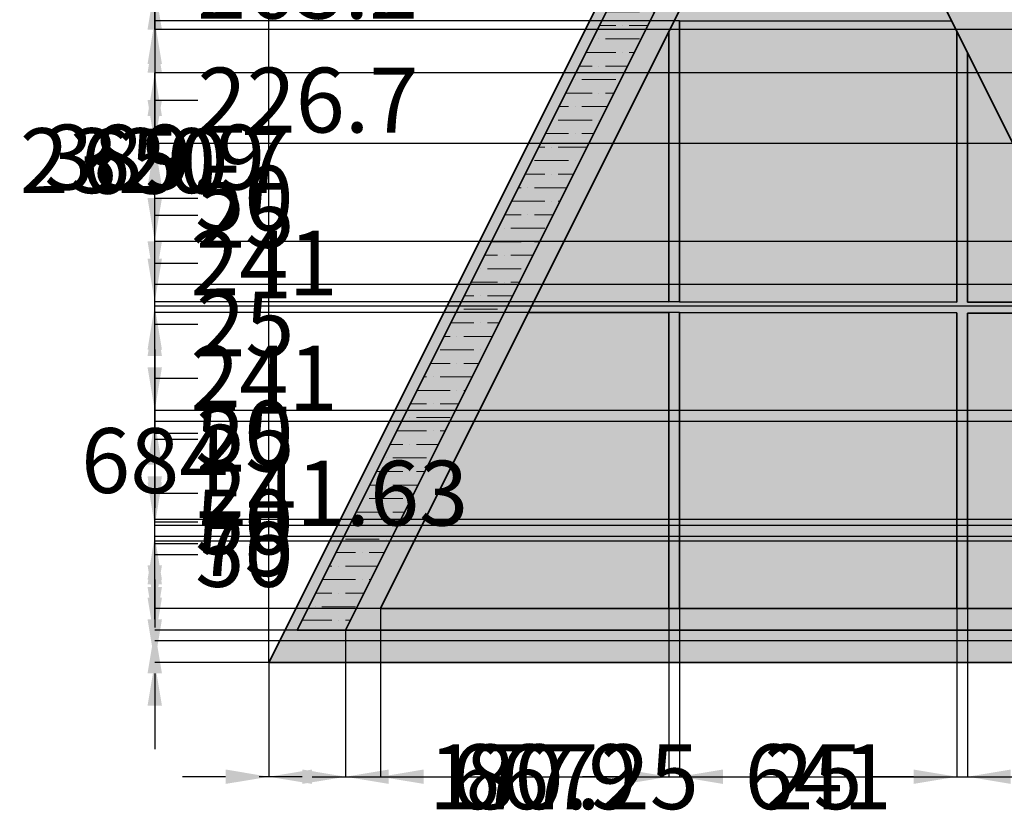
# Model space of a CAD drawing. Units: millimetres. Extents: x -504 to 6314, y 1290 to 4335.
# Tile 1 of 9: x -504 to 1774, y 1290 to 3138. Entities that reach past the tile are written whole.
import ezdxf

# ---------------------------------------------------------------- set-up
doc = ezdxf.new("R2010")
doc.units = ezdxf.units.MM
doc.header["$MEASUREMENT"] = 0
for name, color, linetype, lineweight in [('A-ANNO-DIMS', 2, 'Continuous', 18), ('A-ELEV', 7, 'Continuous', 35), ('A-ELEV-PATT', 8, 'Continuous', 13)]:
    doc.layers.add(name, color=color, linetype=linetype, lineweight=lineweight)
doc.styles.get("Standard").update_dxf_attribs({"font": 'arial.ttf'})
doc.dimstyles.get("Standard").update_dxf_attribs({"dimtxt": 150, "dimasz": 100, "dimexe": 0.18, "dimexo": 0.0625, "dimgap": 0.09, "dimtad": 0, "dimtih": 1, "dimtoh": 1, "dimdec": 0, "dimzin": 0, "dimdsep": 46, "dimtxsty": 'Standard', "dimcen": 0.09, "dimadec": 0, "dimazin": 0, "dimtfac": 1, "dimtdec": 0, "dimtofl": 0, "dimtmove": 0, "dimatfit": 3, "dimfxl": 1, "dimtolj": 1, "dimtzin": 0, "dimarcsym": 0})

# ---------------------------------------------------------------- blocks, each defined once
blk = doc.blocks.new('*D1')
at = {"layer": 'A-ANNO-DIMS', "color": 0, "lineweight": -2, "transparency": 16777216}
for p, q in [((5324.8, 2261.1), (5324.8, 1387.9)), ((72.8, 1652.1), (72.8, 1387.9)), ((172.8, 1388.1), (2475.5, 1388.1)), ((5224.8, 1388.1), (2922.1, 1388.1))]:
    blk.add_line(p, q, dxfattribs=at)
at = {"layer": 'A-ANNO-DIMS', "color": 0, "transparency": 16777216}
for points in [[(172.8, 1404.8), (172.8, 1371.5), (72.8, 1388.1)], [(5224.8, 1404.8), (5224.8, 1371.5), (5324.8, 1388.1)]]:
    blk.add_solid(points, dxfattribs=at)
at = {"layer": 'Defpoints', "color": 0, "transparency": 16777216}
for p in [(5324.8, 2261.2), (72.8, 1652.1), (5324.8, 1388.1)]:
    blk.add_point(p, dxfattribs=at)
at = {"layer": 'A-ANNO-DIMS', "color": 0, "transparency": 16777216, "insert": (2698.8, 1388.1), "char_height": 150, "attachment_point": 5}
blk.add_mtext('\\A1;5252', dxfattribs=at)
blk = doc.blocks.new('*D2')
at = {"layer": 'A-ANNO-DIMS', "color": 0, "lineweight": -2, "transparency": 16777216}
for p, q in [((1233.1, 3972.8), (-191.3, 3972.8)), ((-191.2, 3872.8), (-191.2, 2889.2)), ((-191.2, 1752.1), (-191.2, 2735.7)), ((72.8, 1652.1), (-191.3, 1652.1))]:
    blk.add_line(p, q, dxfattribs=at)
at = {"layer": 'A-ANNO-DIMS', "color": 0, "transparency": 16777216}
for points in [[(-207.8, 3872.8), (-174.5, 3872.8), (-191.2, 3972.8)], [(-207.8, 1752.1), (-174.5, 1752.1), (-191.2, 1652.1)]]:
    blk.add_solid(points, dxfattribs=at)
at = {"layer": 'Defpoints', "color": 0, "transparency": 16777216}
for p in [(-191.2, 3972.8), (1233.2, 3972.8), (72.8, 1652.1)]:
    blk.add_point(p, dxfattribs=at)
at = {"layer": 'A-ANNO-DIMS', "color": 0, "transparency": 16777216, "insert": (-191.2, 2812.5), "char_height": 150, "attachment_point": 5}
blk.add_mtext('\\A1;2320.7', dxfattribs=at)
blk = doc.blocks.new('*D3')
at = {"layer": 'A-ANNO-DIMS', "color": 0, "lineweight": -2, "transparency": 16777216}
for p, q in [((72.8, 1652.2), (72.8, 4237)), ((172.8, 4236.8), (348.6, 4236.8)), ((1133.2, 4236.8), (957.4, 4236.8)), ((1233.2, 3972.8), (1233.2, 4237))]:
    blk.add_line(p, q, dxfattribs=at)
at = {"layer": 'A-ANNO-DIMS', "color": 0, "transparency": 16777216}
for points in [[(172.8, 4253.4), (172.8, 4220.1), (72.8, 4236.8)], [(1133.2, 4253.4), (1133.2, 4220.1), (1233.2, 4236.8)]]:
    blk.add_solid(points, dxfattribs=at)
at = {"layer": 'Defpoints', "color": 0, "transparency": 16777216}
for p in [(1233.2, 4236.8), (1233.2, 3972.8), (72.8, 1652.1)]:
    blk.add_point(p, dxfattribs=at)
at = {"layer": 'A-ANNO-DIMS', "color": 0, "transparency": 16777216, "insert": (653, 4236.8), "char_height": 150, "attachment_point": 5}
blk.add_mtext('\\A1;1160.3', dxfattribs=at)
blk = doc.blocks.new('*D5')
at = {"layer": 'A-ANNO-DIMS', "color": 0, "lineweight": -2, "transparency": 16777216}
for p, q in [((4260.1, 2625.8), (5589, 2625.8)), ((5588.8, 2525.8), (5588.8, 2215.7)), ((5588.8, 1752.1), (5588.8, 2062.2)), ((72.9, 1652.1), (5589, 1652.1))]:
    blk.add_line(p, q, dxfattribs=at)
at = {"layer": 'A-ANNO-DIMS', "color": 0, "transparency": 16777216}
for points in [[(5572.1, 2525.8), (5605.5, 2525.8), (5588.8, 2625.8)], [(5572.1, 1752.1), (5605.5, 1752.1), (5588.8, 1652.1)]]:
    blk.add_solid(points, dxfattribs=at)
at = {"layer": 'Defpoints', "color": 0, "transparency": 16777216}
for p in [(4260, 2625.8), (5588.8, 2625.8), (72.8, 1652.1)]:
    blk.add_point(p, dxfattribs=at)
at = {"layer": 'A-ANNO-DIMS', "color": 0, "transparency": 16777216, "insert": (5588.8, 2138.9), "char_height": 150, "attachment_point": 5}
blk.add_mtext('\\A1;973.6', dxfattribs=at)
blk = doc.blocks.new('*D6')
at = {"layer": 'A-ANNO-DIMS', "color": 0, "lineweight": -2, "transparency": 16777216}
for p, q in [((72.8, 1652.2), (72.8, 4237)), ((172.8, 4236.8), (920.4, 4236.8)), ((2293.5, 4236.8), (1545.9, 4236.8)), ((2393.5, 1652.2), (2393.5, 4237))]:
    blk.add_line(p, q, dxfattribs=at)
at = {"layer": 'A-ANNO-DIMS', "color": 0, "transparency": 16777216}
for points in [[(172.8, 4253.4), (172.8, 4220.1), (72.8, 4236.8)], [(2293.5, 4253.4), (2293.5, 4220.1), (2393.5, 4236.8)]]:
    blk.add_solid(points, dxfattribs=at)
at = {"layer": 'Defpoints', "color": 0, "transparency": 16777216}
for p in [(2393.5, 4236.8), (72.8, 1652.1), (2393.5, 1652.1)]:
    blk.add_point(p, dxfattribs=at)
at = {"layer": 'A-ANNO-DIMS', "color": 0, "transparency": 16777216, "insert": (1233.2, 4236.8), "char_height": 150, "attachment_point": 5}
blk.add_mtext('\\A1;2320.7', dxfattribs=at)
blk = doc.blocks.new('*D7')
at = {"layer": 'A-ANNO-DIMS', "color": 0, "lineweight": -2, "transparency": 16777216}
for p, q in [((250.1, 1727.1), (250.1, 1387.9)), ((72.8, 1652.1), (72.8, 1387.9)), ((-27.2, 1388.1), (-127.2, 1388.1)), ((350.1, 1388.1), (450.1, 1388.1))]:
    blk.add_line(p, q, dxfattribs=at)
at = {"layer": 'A-ANNO-DIMS', "color": 0, "transparency": 16777216}
for points in [[(-27.2, 1404.8), (-27.2, 1371.5), (72.8, 1388.1)], [(350.1, 1404.8), (350.1, 1371.5), (250.1, 1388.1)]]:
    blk.add_solid(points, dxfattribs=at)
at = {"layer": 'Defpoints', "color": 0, "transparency": 16777216}
for p in [(250.1, 1727.1), (72.8, 1652.1), (250.1, 1388.1)]:
    blk.add_point(p, dxfattribs=at)
at = {"layer": 'A-ANNO-DIMS', "color": 0, "transparency": 16777216, "insert": (755, 1388.1), "char_height": 150, "attachment_point": 5}
blk.add_mtext('\\A1;177.25', dxfattribs=at)
blk = doc.blocks.new('*D8')
at = {"layer": 'A-ANNO-DIMS', "color": 0, "lineweight": -2, "transparency": 16777216}
for p, q in [((331, 1777.1), (331, 1387.9)), ((250.1, 1727.1), (250.1, 1387.9)), ((150.1, 1388.1), (50.1, 1388.1)), ((431, 1388.1), (531, 1388.1))]:
    blk.add_line(p, q, dxfattribs=at)
at = {"layer": 'A-ANNO-DIMS', "color": 0, "transparency": 16777216}
for points in [[(150.1, 1404.8), (150.1, 1371.5), (250.1, 1388.1)], [(431, 1404.8), (431, 1371.5), (331, 1388.1)]]:
    blk.add_solid(points, dxfattribs=at)
at = {"layer": 'Defpoints', "color": 0, "transparency": 16777216}
for p in [(331, 1777.1), (250.1, 1727.1), (331, 1388.1)]:
    blk.add_point(p, dxfattribs=at)
at = {"layer": 'A-ANNO-DIMS', "color": 0, "transparency": 16777216, "insert": (726.2, 1388.1), "char_height": 150, "attachment_point": 5}
blk.add_mtext('\\A1;80.9', dxfattribs=at)
blk = doc.blocks.new('*D9')
at = {"layer": 'A-ANNO-DIMS', "color": 0, "lineweight": -2, "transparency": 16777216}
for p, q in [((331, 1777.1), (331, 1387.9)), ((998, 1777.1), (998, 1387.9)), ((431, 1388.1), (498.3, 1388.1)), ((898, 1388.1), (830.7, 1388.1))]:
    blk.add_line(p, q, dxfattribs=at)
at = {"layer": 'A-ANNO-DIMS', "color": 0, "transparency": 16777216}
for points in [[(431, 1404.8), (431, 1371.5), (331, 1388.1)], [(898, 1404.8), (898, 1371.5), (998, 1388.1)]]:
    blk.add_solid(points, dxfattribs=at)
at = {"layer": 'Defpoints', "color": 0, "transparency": 16777216}
for p in [(331, 1777.1), (998, 1777.1), (998, 1388.1)]:
    blk.add_point(p, dxfattribs=at)
at = {"layer": 'A-ANNO-DIMS', "color": 0, "transparency": 16777216, "insert": (664.5, 1388.1), "char_height": 150, "attachment_point": 5}
blk.add_mtext('\\A1;667', dxfattribs=at)
blk = doc.blocks.new('*D10')
at = {"layer": 'A-ANNO-DIMS', "color": 0, "lineweight": -2, "transparency": 16777216}
for p, q in [((998, 1777.1), (998, 1387.9)), ((1023, 1777.1), (1023, 1387.9)), ((898, 1388.1), (798, 1388.1)), ((1123, 1388.1), (1223, 1388.1))]:
    blk.add_line(p, q, dxfattribs=at)
at = {"layer": 'A-ANNO-DIMS', "color": 0, "transparency": 16777216}
for points in [[(898, 1404.8), (898, 1371.5), (998, 1388.1)], [(1123, 1404.8), (1123, 1371.5), (1023, 1388.1)]]:
    blk.add_solid(points, dxfattribs=at)
at = {"layer": 'Defpoints', "color": 0, "transparency": 16777216}
for p in [(998, 1777.1), (1023, 1777.1), (1023, 1388.1)]:
    blk.add_point(p, dxfattribs=at)
at = {"layer": 'A-ANNO-DIMS', "color": 0, "transparency": 16777216, "insert": (1332.4, 1388.1), "char_height": 150, "attachment_point": 5}
blk.add_mtext('\\A1;25', dxfattribs=at)
blk = doc.blocks.new('*D11')
at = {"layer": 'A-ANNO-DIMS', "color": 0, "lineweight": -2, "transparency": 16777216}
for p, q in [((1023, 1777.1), (1023, 1387.9)), ((1664, 1777.1), (1664, 1387.9)), ((1123, 1388.1), (1191.8, 1388.1)), ((1564, 1388.1), (1495.2, 1388.1))]:
    blk.add_line(p, q, dxfattribs=at)
at = {"layer": 'A-ANNO-DIMS', "color": 0, "transparency": 16777216}
for points in [[(1123, 1404.8), (1123, 1371.5), (1023, 1388.1)], [(1564, 1404.8), (1564, 1371.5), (1664, 1388.1)]]:
    blk.add_solid(points, dxfattribs=at)
at = {"layer": 'Defpoints', "color": 0, "transparency": 16777216}
for p in [(1023, 1777.1), (1664, 1777.1), (1664, 1388.1)]:
    blk.add_point(p, dxfattribs=at)
at = {"layer": 'A-ANNO-DIMS', "color": 0, "transparency": 16777216, "insert": (1343.5, 1388.1), "char_height": 150, "attachment_point": 5}
blk.add_mtext('\\A1;641', dxfattribs=at)
blk = doc.blocks.new('*D12')
at = {"layer": 'A-ANNO-DIMS', "color": 0, "lineweight": -2, "transparency": 16777216}
for p, q in [((1664, 1777.1), (1664, 1387.9)), ((1689, 1777.1), (1689, 1387.9)), ((1564, 1388.1), (1464, 1388.1)), ((1789, 1388.1), (1889, 1388.1))]:
    blk.add_line(p, q, dxfattribs=at)
at = {"layer": 'A-ANNO-DIMS', "color": 0, "transparency": 16777216}
for points in [[(1564, 1404.8), (1564, 1371.5), (1664, 1388.1)], [(1789, 1404.8), (1789, 1371.5), (1689, 1388.1)]]:
    blk.add_solid(points, dxfattribs=at)
at = {"layer": 'Defpoints', "color": 0, "transparency": 16777216}
for p in [(1664, 1777.1), (1689, 1777.1), (1689, 1388.1)]:
    blk.add_point(p, dxfattribs=at)
at = {"layer": 'A-ANNO-DIMS', "color": 0, "transparency": 16777216, "insert": (1998.4, 1388.1), "char_height": 150, "attachment_point": 5}
blk.add_mtext('\\A1;25', dxfattribs=at)
blk = doc.blocks.new('*D13')
at = {"layer": 'A-ANNO-DIMS', "color": 0, "lineweight": -2, "transparency": 16777216}
for p, q in [((1689, 1777.1), (1689, 1387.9)), ((2331, 1777.1), (2331, 1387.9)), ((1789, 1388.1), (1844.6, 1388.1)), ((2231, 1388.1), (2175.4, 1388.1))]:
    blk.add_line(p, q, dxfattribs=at)
at = {"layer": 'A-ANNO-DIMS', "color": 0, "transparency": 16777216}
for points in [[(1789, 1404.8), (1789, 1371.5), (1689, 1388.1)], [(2231, 1404.8), (2231, 1371.5), (2331, 1388.1)]]:
    blk.add_solid(points, dxfattribs=at)
at = {"layer": 'Defpoints', "color": 0, "transparency": 16777216}
for p in [(1689, 1777.1), (2331, 1777.1), (2331, 1388.1)]:
    blk.add_point(p, dxfattribs=at)
at = {"layer": 'A-ANNO-DIMS', "color": 0, "transparency": 16777216, "insert": (2010, 1388.1), "char_height": 150, "attachment_point": 5}
blk.add_mtext('\\A1;642', dxfattribs=at)
blk = doc.blocks.new('*D14')
at = {"layer": 'A-ANNO-DIMS', "color": 0, "lineweight": -2, "transparency": 16777216}
for p, q in [((-191.2, 1827.1), (-191.2, 1927.1)), ((-191.2, 1927.1), (-91.2, 1927.1)), ((138.2, 1727.1), (-191.3, 1727.1)), ((72.8, 1652.1), (-191.3, 1652.1)), ((-191.2, 1552.1), (-191.2, 1452.1))]:
    blk.add_line(p, q, dxfattribs=at)
at = {"layer": 'A-ANNO-DIMS', "color": 0, "transparency": 16777216}
for points in [[(-207.8, 1827.1), (-174.5, 1827.1), (-191.2, 1727.1)], [(-207.8, 1552.1), (-174.5, 1552.1), (-191.2, 1652.1)]]:
    blk.add_solid(points, dxfattribs=at)
at = {"layer": 'Defpoints', "color": 0, "transparency": 16777216}
for p in [(-191.2, 1727.1), (138.3, 1727.1), (72.8, 1652.1)]:
    blk.add_point(p, dxfattribs=at)
at = {"layer": 'A-ANNO-DIMS', "color": 0, "transparency": 16777216, "insert": (16.3, 1927.1), "char_height": 150, "attachment_point": 5}
blk.add_mtext('\\A1;75', dxfattribs=at)
blk = doc.blocks.new('*D15')
at = {"layer": 'A-ANNO-DIMS', "color": 0, "lineweight": -2, "transparency": 16777216}
for p, q in [((-191.2, 1877.1), (-191.2, 1977.1)), ((-191.2, 1977.1), (-91.2, 1977.1)), ((330.9, 1777.1), (-191.3, 1777.1)), ((138.2, 1727.1), (-191.3, 1727.1)), ((-191.2, 1627.1), (-191.2, 1527.1))]:
    blk.add_line(p, q, dxfattribs=at)
at = {"layer": 'A-ANNO-DIMS', "color": 0, "transparency": 16777216}
for points in [[(-207.8, 1877.1), (-174.5, 1877.1), (-191.2, 1777.1)], [(-207.8, 1627.1), (-174.5, 1627.1), (-191.2, 1727.1)]]:
    blk.add_solid(points, dxfattribs=at)
at = {"layer": 'Defpoints', "color": 0, "transparency": 16777216}
for p in [(-191.2, 1777.1), (331, 1777.1), (138.3, 1727.1)]:
    blk.add_point(p, dxfattribs=at)
at = {"layer": 'A-ANNO-DIMS', "color": 0, "transparency": 16777216, "insert": (16.1, 1977.1), "char_height": 150, "attachment_point": 5}
blk.add_mtext('\\A1;50', dxfattribs=at)
blk = doc.blocks.new('*D16')
at = {"layer": 'A-ANNO-DIMS', "color": 0, "lineweight": -2, "transparency": 16777216}
for p, q in [((1022.9, 2461.1), (-191.3, 2461.1)), ((-191.2, 2361.1), (-191.2, 2195.8)), ((-191.2, 1877.1), (-191.2, 2042.4)), ((1022.9, 1777.1), (-191.3, 1777.1))]:
    blk.add_line(p, q, dxfattribs=at)
at = {"layer": 'A-ANNO-DIMS', "color": 0, "transparency": 16777216}
for points in [[(-207.8, 2361.1), (-174.5, 2361.1), (-191.2, 2461.1)], [(-207.8, 1877.1), (-174.5, 1877.1), (-191.2, 1777.1)]]:
    blk.add_solid(points, dxfattribs=at)
at = {"layer": 'Defpoints', "color": 0, "transparency": 16777216}
for p in [(-191.2, 2461.1), (1023, 2461.1), (1023, 1777.1)]:
    blk.add_point(p, dxfattribs=at)
at = {"layer": 'A-ANNO-DIMS', "color": 0, "transparency": 16777216, "insert": (-191.2, 2119.1), "char_height": 150, "attachment_point": 5}
blk.add_mtext('\\A1;684', dxfattribs=at)
blk = doc.blocks.new('*D17')
at = {"layer": 'A-ANNO-DIMS', "color": 0, "lineweight": -2, "transparency": 16777216}
for p, q in [((-191.2, 2586.1), (-191.2, 2686.1)), ((-191.2, 2686.1), (-91.2, 2686.1)), ((1022.9, 2486.1), (-191.3, 2486.1)), ((1022.9, 2461.1), (-191.3, 2461.1)), ((-191.2, 2361.1), (-191.2, 2261.1))]:
    blk.add_line(p, q, dxfattribs=at)
at = {"layer": 'A-ANNO-DIMS', "color": 0, "transparency": 16777216}
for points in [[(-207.8, 2586.1), (-174.5, 2586.1), (-191.2, 2486.1)], [(-207.8, 2361.1), (-174.5, 2361.1), (-191.2, 2461.1)]]:
    blk.add_solid(points, dxfattribs=at)
at = {"layer": 'Defpoints', "color": 0, "transparency": 16777216}
for p in [(-191.2, 2486.1), (1023, 2486.1), (1023, 2461.1)]:
    blk.add_point(p, dxfattribs=at)
at = {"layer": 'A-ANNO-DIMS', "color": 0, "transparency": 16777216, "insert": (18.2, 2686.1), "char_height": 150, "attachment_point": 5}
blk.add_mtext('\\A1;25', dxfattribs=at)
blk = doc.blocks.new('*D18')
at = {"layer": 'A-ANNO-DIMS', "color": 0, "lineweight": -2, "transparency": 16777216}
for p, q in [((1022.9, 3136.1), (-191.3, 3136.1)), ((-191.2, 3036.1), (-191.2, 2887.8)), ((-191.2, 2586.1), (-191.2, 2734.4)), ((1022.9, 2486.1), (-191.3, 2486.1))]:
    blk.add_line(p, q, dxfattribs=at)
at = {"layer": 'A-ANNO-DIMS', "color": 0, "transparency": 16777216}
for points in [[(-207.8, 3036.1), (-174.5, 3036.1), (-191.2, 3136.1)], [(-207.8, 2586.1), (-174.5, 2586.1), (-191.2, 2486.1)]]:
    blk.add_solid(points, dxfattribs=at)
at = {"layer": 'Defpoints', "color": 0, "transparency": 16777216}
for p in [(-191.2, 3136.1), (1023, 3136.1), (1023, 2486.1)]:
    blk.add_point(p, dxfattribs=at)
at = {"layer": 'A-ANNO-DIMS', "color": 0, "transparency": 16777216, "insert": (-191.2, 2811.1), "char_height": 150, "attachment_point": 5}
blk.add_mtext('\\A1;650', dxfattribs=at)
blk = doc.blocks.new('*D19')
at = {"layer": 'A-ANNO-DIMS', "color": 0, "lineweight": -2, "transparency": 16777216}
for p, q in [((-191.2, 3261.1), (-191.2, 3361.1)), ((-191.2, 3361.1), (-91.2, 3361.1)), ((1022.9, 3161.1), (-191.3, 3161.1)), ((1022.9, 3136.1), (-191.3, 3136.1)), ((-191.2, 3036.1), (-191.2, 2936.1))]:
    blk.add_line(p, q, dxfattribs=at)
at = {"layer": 'A-ANNO-DIMS', "color": 0, "transparency": 16777216}
for points in [[(-207.8, 3261.1), (-174.5, 3261.1), (-191.2, 3161.1)], [(-207.8, 3036.1), (-174.5, 3036.1), (-191.2, 3136.1)]]:
    blk.add_solid(points, dxfattribs=at)
at = {"layer": 'Defpoints', "color": 0, "transparency": 16777216}
for p in [(-191.2, 3161.1), (1023, 3161.1), (1023, 3136.1)]:
    blk.add_point(p, dxfattribs=at)
at = {"layer": 'A-ANNO-DIMS', "color": 0, "transparency": 16777216, "insert": (18.2, 3361.1), "char_height": 150, "attachment_point": 5}
blk.add_mtext('\\A1;25', dxfattribs=at)
blk = doc.blocks.new('*D31')
at = {"layer": 'A-ANNO-DIMS', "color": 0, "lineweight": -2, "transparency": 16777216}
for p, q in [((-191.2, 2852.5), (-191.2, 2952.5)), ((-191.2, 2952.5), (-91.2, 2952.5)), ((2963.6, 2852.5), (-191.3, 2852.5)), ((-191.2, 2725.8), (-191.2, 2752.5)), ((2963.6, 2625.8), (-191.3, 2625.8))]:
    blk.add_line(p, q, dxfattribs=at)
at = {"layer": 'A-ANNO-DIMS', "color": 0, "transparency": 16777216}
for points in [[(-207.8, 2752.5), (-174.5, 2752.5), (-191.2, 2852.5)], [(-207.8, 2725.8), (-174.5, 2725.8), (-191.2, 2625.8)]]:
    blk.add_solid(points, dxfattribs=at)
at = {"layer": 'Defpoints', "color": 0, "transparency": 16777216}
for p in [(-191.2, 2852.5), (2963.6, 2852.5), (2963.6, 2625.8)]:
    blk.add_point(p, dxfattribs=at)
at = {"layer": 'A-ANNO-DIMS', "color": 0, "transparency": 16777216, "insert": (163.3, 2952.5), "char_height": 150, "attachment_point": 5}
blk.add_mtext('\\A1;226.7', dxfattribs=at)
blk = doc.blocks.new('*D32')
at = {"layer": 'A-ANNO-DIMS', "color": 0, "lineweight": -2, "transparency": 16777216}
for p, q in [((-191.2, 3115.7), (-191.2, 3215.7)), ((-191.2, 3215.7), (-91.2, 3215.7)), ((2963.6, 3115.7), (-191.3, 3115.7)), ((-191.2, 2952.5), (-191.2, 3015.7)), ((2963.6, 2852.5), (-191.3, 2852.5))]:
    blk.add_line(p, q, dxfattribs=at)
at = {"layer": 'A-ANNO-DIMS', "color": 0, "transparency": 16777216}
for points in [[(-207.8, 3015.7), (-174.5, 3015.7), (-191.2, 3115.7)], [(-207.8, 2952.5), (-174.5, 2952.5), (-191.2, 2852.5)]]:
    blk.add_solid(points, dxfattribs=at)
at = {"layer": 'Defpoints', "color": 0, "transparency": 16777216}
for p in [(-191.2, 3115.7), (2963.6, 3115.7), (2963.6, 2852.5)]:
    blk.add_point(p, dxfattribs=at)
at = {"layer": 'A-ANNO-DIMS', "color": 0, "transparency": 16777216, "insert": (162.5, 3215.7), "char_height": 150, "attachment_point": 5}
blk.add_mtext('\\A1;263.2', dxfattribs=at)
blk = doc.blocks.new('*D33')
at = {"layer": 'A-ANNO-DIMS', "color": 0, "lineweight": -2, "transparency": 16777216}
for p, q in [((-191.2, 3315.7), (-191.2, 3415.7)), ((-191.2, 3415.7), (-91.2, 3415.7)), ((2963.6, 3215.7), (-191.3, 3215.7)), ((2963.6, 3115.7), (-191.3, 3115.7)), ((-191.2, 3015.7), (-191.2, 2915.7))]:
    blk.add_line(p, q, dxfattribs=at)
at = {"layer": 'A-ANNO-DIMS', "color": 0, "transparency": 16777216}
for points in [[(-207.8, 3315.7), (-174.5, 3315.7), (-191.2, 3215.7)], [(-207.8, 3015.7), (-174.5, 3015.7), (-191.2, 3115.7)]]:
    blk.add_solid(points, dxfattribs=at)
at = {"layer": 'Defpoints', "color": 0, "transparency": 16777216}
for p in [(-191.2, 3215.7), (2963.6, 3215.7), (2963.6, 3115.7)]:
    blk.add_point(p, dxfattribs=at)
at = {"layer": 'A-ANNO-DIMS', "color": 0, "transparency": 16777216, "insert": (67.3, 3415.7), "char_height": 150, "attachment_point": 5}
blk.add_mtext('\\A1;100', dxfattribs=at)
blk = doc.blocks.new('*D34')
at = {"layer": 'A-ANNO-DIMS', "color": 0, "lineweight": -2, "transparency": 16777216}
for p, q in [((-191.2, 3390.7), (-191.2, 3490.7)), ((-191.2, 3490.7), (-91.2, 3490.7)), ((2963.6, 3290.7), (-191.3, 3290.7)), ((2963.6, 3215.7), (-191.3, 3215.7)), ((-191.2, 3115.7), (-191.2, 3015.7))]:
    blk.add_line(p, q, dxfattribs=at)
at = {"layer": 'A-ANNO-DIMS', "color": 0, "transparency": 16777216}
for points in [[(-207.8, 3390.7), (-174.5, 3390.7), (-191.2, 3290.7)], [(-207.8, 3115.7), (-174.5, 3115.7), (-191.2, 3215.7)]]:
    blk.add_solid(points, dxfattribs=at)
at = {"layer": 'Defpoints', "color": 0, "transparency": 16777216}
for p in [(-191.2, 3290.7), (2963.6, 3290.7), (2963.6, 3215.7)]:
    blk.add_point(p, dxfattribs=at)
at = {"layer": 'A-ANNO-DIMS', "color": 0, "transparency": 16777216, "insert": (16.3, 3490.7), "char_height": 150, "attachment_point": 5}
blk.add_mtext('\\A1;75', dxfattribs=at)
blk = doc.blocks.new('*D35')
at = {"layer": 'A-ANNO-DIMS', "color": 0, "lineweight": -2, "transparency": 16777216}
for p, q in [((3418.6, 3015.7), (-191.3, 3015.7)), ((-191.2, 2915.7), (-191.2, 2897.4)), ((-191.2, 2725.8), (-191.2, 2744)), ((3407.7, 2625.8), (-191.3, 2625.8))]:
    blk.add_line(p, q, dxfattribs=at)
at = {"layer": 'A-ANNO-DIMS', "color": 0, "transparency": 16777216}
for points in [[(-207.8, 2915.7), (-174.5, 2915.7), (-191.2, 3015.7)], [(-207.8, 2725.8), (-174.5, 2725.8), (-191.2, 2625.8)]]:
    blk.add_solid(points, dxfattribs=at)
at = {"layer": 'Defpoints', "color": 0, "transparency": 16777216}
for p in [(-191.2, 3015.7), (3418.6, 3015.7), (3407.8, 2625.8)]:
    blk.add_point(p, dxfattribs=at)
at = {"layer": 'A-ANNO-DIMS', "color": 0, "transparency": 16777216, "insert": (-191.2, 2820.7), "char_height": 150, "attachment_point": 5}
blk.add_mtext('\\A1;389.9', dxfattribs=at)
blk = doc.blocks.new('*D67')
at = {"layer": 'A-ANNO-DIMS', "color": 0, "lineweight": -2, "transparency": 16777216}
for p, q in [((-191.2, 2082.8), (-191.2, 2182.8)), ((-191.2, 2182.8), (-91.2, 2182.8)), ((3992, 1982.8), (-191.3, 1982.8)), ((3853.6, 1932.8), (-191.3, 1932.8)), ((-191.2, 1832.8), (-191.2, 1732.8))]:
    blk.add_line(p, q, dxfattribs=at)
at = {"layer": 'A-ANNO-DIMS', "color": 0, "transparency": 16777216}
for points in [[(-207.8, 2082.8), (-174.5, 2082.8), (-191.2, 1982.8)], [(-207.8, 1832.8), (-174.5, 1832.8), (-191.2, 1932.8)]]:
    blk.add_solid(points, dxfattribs=at)
at = {"layer": 'Defpoints', "color": 0, "transparency": 16777216}
for p in [(-191.2, 1982.8), (3992.1, 1982.8), (3853.7, 1932.8)]:
    blk.add_point(p, dxfattribs=at)
at = {"layer": 'A-ANNO-DIMS', "color": 0, "transparency": 16777216, "insert": (16.1, 2182.8), "char_height": 150, "attachment_point": 5}
blk.add_mtext('\\A1;50', dxfattribs=at)
blk = doc.blocks.new('*D68')
at = {"layer": 'A-ANNO-DIMS', "color": 0, "lineweight": -2, "transparency": 16777216}
for p, q in [((-191.2, 1802.1), (-191.2, 1902.1)), ((-191.2, 1902.1), (-91.2, 1902.1)), ((3076.9, 1702.1), (-191.3, 1702.1)), ((3076.9, 1652.1), (-191.3, 1652.1)), ((-191.2, 1552.1), (-191.2, 1452.1))]:
    blk.add_line(p, q, dxfattribs=at)
at = {"layer": 'A-ANNO-DIMS', "color": 0, "transparency": 16777216}
for points in [[(-207.8, 1802.1), (-174.5, 1802.1), (-191.2, 1702.1)], [(-207.8, 1552.1), (-174.5, 1552.1), (-191.2, 1652.1)]]:
    blk.add_solid(points, dxfattribs=at)
at = {"layer": 'Defpoints', "color": 0, "transparency": 16777216}
for p in [(-191.2, 1702.1), (3077, 1702.1), (3077, 1652.1)]:
    blk.add_point(p, dxfattribs=at)
at = {"layer": 'A-ANNO-DIMS', "color": 0, "transparency": 16777216, "insert": (16.1, 1902.1), "char_height": 150, "attachment_point": 5}
blk.add_mtext('\\A1;50', dxfattribs=at)
blk = doc.blocks.new('*D69')
at = {"layer": 'A-ANNO-DIMS', "color": 0, "lineweight": -2, "transparency": 16777216}
for p, q in [((-191.2, 2625.8), (-191.2, 2725.8)), ((-191.2, 2725.8), (-91.2, 2725.8)), ((3076.9, 2525.8), (-191.3, 2525.8)), ((3076.9, 2475.8), (-191.3, 2475.8)), ((-191.2, 2375.8), (-191.2, 2275.8))]:
    blk.add_line(p, q, dxfattribs=at)
at = {"layer": 'A-ANNO-DIMS', "color": 0, "transparency": 16777216}
for points in [[(-207.8, 2625.8), (-174.5, 2625.8), (-191.2, 2525.8)], [(-207.8, 2375.8), (-174.5, 2375.8), (-191.2, 2475.8)]]:
    blk.add_solid(points, dxfattribs=at)
at = {"layer": 'Defpoints', "color": 0, "transparency": 16777216}
for p in [(-191.2, 2525.8), (3077, 2525.8), (3077, 2475.8)]:
    blk.add_point(p, dxfattribs=at)
at = {"layer": 'A-ANNO-DIMS', "color": 0, "transparency": 16777216, "insert": (16.1, 2725.8), "char_height": 150, "attachment_point": 5}
blk.add_mtext('\\A1;50', dxfattribs=at)
blk = doc.blocks.new('*D70')
at = {"layer": 'A-ANNO-DIMS', "color": 0, "lineweight": -2, "transparency": 16777216}
for p, q in [((-191.2, 1943.8), (-191.2, 2043.8)), ((-191.2, 2043.8), (-91.2, 2043.8)), ((3447.7, 1943.8), (-191.3, 1943.8)), ((-191.2, 1802.1), (-191.2, 1843.8)), ((3447.7, 1702.1), (-191.3, 1702.1))]:
    blk.add_line(p, q, dxfattribs=at)
at = {"layer": 'A-ANNO-DIMS', "color": 0, "transparency": 16777216}
for points in [[(-207.8, 1843.8), (-174.5, 1843.8), (-191.2, 1943.8)], [(-207.8, 1802.1), (-174.5, 1802.1), (-191.2, 1702.1)]]:
    blk.add_solid(points, dxfattribs=at)
at = {"layer": 'Defpoints', "color": 0, "transparency": 16777216}
for p in [(-191.2, 1943.8), (3447.8, 1943.8), (3447.8, 1702.1)]:
    blk.add_point(p, dxfattribs=at)
at = {"layer": 'A-ANNO-DIMS', "color": 0, "transparency": 16777216, "insert": (221.6, 2043.8), "char_height": 150, "attachment_point": 5}
blk.add_mtext('\\A1;241.63', dxfattribs=at)
blk = doc.blocks.new('*D71')
at = {"layer": 'A-ANNO-DIMS', "color": 0, "lineweight": -2, "transparency": 16777216}
for p, q in [((-191.2, 2068.8), (-191.2, 2168.8)), ((-191.2, 2168.8), (-91.2, 2168.8)), ((3447.7, 1968.8), (-191.3, 1968.8)), ((3447.7, 1943.8), (-191.3, 1943.8)), ((-191.2, 1843.8), (-191.2, 1743.8))]:
    blk.add_line(p, q, dxfattribs=at)
at = {"layer": 'A-ANNO-DIMS', "color": 0, "transparency": 16777216}
for points in [[(-207.8, 2068.8), (-174.5, 2068.8), (-191.2, 1968.8)], [(-207.8, 1843.8), (-174.5, 1843.8), (-191.2, 1943.8)]]:
    blk.add_solid(points, dxfattribs=at)
at = {"layer": 'Defpoints', "color": 0, "transparency": 16777216}
for p in [(-191.2, 1968.8), (3447.8, 1968.8), (3447.8, 1943.8)]:
    blk.add_point(p, dxfattribs=at)
at = {"layer": 'A-ANNO-DIMS', "color": 0, "transparency": 16777216, "insert": (18.2, 2168.8), "char_height": 150, "attachment_point": 5}
blk.add_mtext('\\A1;25', dxfattribs=at)
blk = doc.blocks.new('*D72')
at = {"layer": 'A-ANNO-DIMS', "color": 0, "lineweight": -2, "transparency": 16777216}
for p, q in [((-191.2, 2209.8), (-191.2, 2309.8)), ((-191.2, 2309.8), (-91.2, 2309.8)), ((3447.7, 2209.8), (-191.3, 2209.8)), ((-191.2, 2068.8), (-191.2, 2109.8)), ((3447.7, 1968.8), (-191.3, 1968.8))]:
    blk.add_line(p, q, dxfattribs=at)
at = {"layer": 'A-ANNO-DIMS', "color": 0, "transparency": 16777216}
for points in [[(-207.8, 2109.8), (-174.5, 2109.8), (-191.2, 2209.8)], [(-207.8, 2068.8), (-174.5, 2068.8), (-191.2, 1968.8)]]:
    blk.add_solid(points, dxfattribs=at)
at = {"layer": 'Defpoints', "color": 0, "transparency": 16777216}
for p in [(-191.2, 2209.8), (3447.8, 2209.8), (3447.8, 1968.8)]:
    blk.add_point(p, dxfattribs=at)
at = {"layer": 'A-ANNO-DIMS', "color": 0, "transparency": 16777216, "insert": (61.4, 2309.8), "char_height": 150, "attachment_point": 5}
blk.add_mtext('\\A1;241', dxfattribs=at)
blk = doc.blocks.new('*D73')
at = {"layer": 'A-ANNO-DIMS', "color": 0, "lineweight": -2, "transparency": 16777216}
for p, q in [((-191.2, 2334.8), (-191.2, 2434.8)), ((-191.2, 2434.8), (-91.2, 2434.8)), ((3447.7, 2234.8), (-191.3, 2234.8)), ((3447.7, 2209.8), (-191.3, 2209.8)), ((-191.2, 2109.8), (-191.2, 2009.8))]:
    blk.add_line(p, q, dxfattribs=at)
at = {"layer": 'A-ANNO-DIMS', "color": 0, "transparency": 16777216}
for points in [[(-207.8, 2334.8), (-174.5, 2334.8), (-191.2, 2234.8)], [(-207.8, 2109.8), (-174.5, 2109.8), (-191.2, 2209.8)]]:
    blk.add_solid(points, dxfattribs=at)
at = {"layer": 'Defpoints', "color": 0, "transparency": 16777216}
for p in [(-191.2, 2234.8), (3447.8, 2234.8), (3447.8, 2209.8)]:
    blk.add_point(p, dxfattribs=at)
at = {"layer": 'A-ANNO-DIMS', "color": 0, "transparency": 16777216, "insert": (18.2, 2434.8), "char_height": 150, "attachment_point": 5}
blk.add_mtext('\\A1;25', dxfattribs=at)
blk = doc.blocks.new('*D74')
at = {"layer": 'A-ANNO-DIMS', "color": 0, "lineweight": -2, "transparency": 16777216}
for p, q in [((-191.2, 2475.8), (-191.2, 2575.8)), ((-191.2, 2575.8), (-91.2, 2575.8)), ((3447.7, 2475.8), (-191.3, 2475.8)), ((-191.2, 2334.8), (-191.2, 2375.8)), ((3447.7, 2234.8), (-191.3, 2234.8))]:
    blk.add_line(p, q, dxfattribs=at)
at = {"layer": 'A-ANNO-DIMS', "color": 0, "transparency": 16777216}
for points in [[(-207.8, 2375.8), (-174.5, 2375.8), (-191.2, 2475.8)], [(-207.8, 2334.8), (-174.5, 2334.8), (-191.2, 2234.8)]]:
    blk.add_solid(points, dxfattribs=at)
at = {"layer": 'Defpoints', "color": 0, "transparency": 16777216}
for p in [(-191.2, 2475.8), (3447.8, 2475.8), (3447.8, 2234.8)]:
    blk.add_point(p, dxfattribs=at)
at = {"layer": 'A-ANNO-DIMS', "color": 0, "transparency": 16777216, "insert": (61.4, 2575.8), "char_height": 150, "attachment_point": 5}
blk.add_mtext('\\A1;241', dxfattribs=at)

msp = doc.modelspace()

# ---------------------------------------------------------------- hatches: boundary and pattern name
at = {"layer": 'A-ELEV-PATT'}
for points in [[(3324.48, 3780.626), (1233.163, 3972.781), (72.835, 1652.125), (2393.491, 1652.125), (2355.991, 1727.125), (138.286, 1727.125), (1247.138, 3944.83), (2393.491, 1652.125), (2840.705, 1652.125), (2403.888, 2525.758), (2236.182, 2525.758), (2186.182, 2625.758), (2309.166, 2625.758), (1976.702, 3290.687), (1853.718, 3290.687), (1778.718, 3440.687), (3407.797, 3440.687)], [(1303.04, 3833.026), (1247.138, 3944.83), (138.286, 1727.125), (250.089, 1727.125)], [(1330.991, 3777.125), (1303.04, 3833.026), (250.089, 1727.125), (2355.991, 1727.125), (2330.991, 1777.125), (330.991, 1777.125)], [(1977.097, 2484.912), (1688.991, 2485.278), (1688.991, 3061.125), (1663.991, 3111.125), (1663.991, 2485.31), (1022.991, 2486.124), (1022.991, 3136.125), (1651.89, 3135.326), (1639.382, 3160.342), (1022.991, 3161.125), (997.991, 3111.125), (997.991, 2486.156), (685.705, 2486.552), (673.213, 2461.568), (997.991, 2461.156), (997.991, 1777.125), (1022.991, 1777.125), (1022.991, 2461.124), (1663.991, 2460.31), (1663.991, 1777.125), (1688.991, 1777.125), (1688.991, 2460.278), (1989.605, 2459.896)]]:
    msp.add_hatch(color=256, dxfattribs=at).paths.add_polyline_path(points)
h = msp.add_hatch(dxfattribs=at)
h.set_pattern_fill('ANSI36', color=256, scale=200, angle=135, style=0)
h.paths.add_polyline_path([(3324.48, 3780.626), (1233.163, 3972.781), (72.835, 1652.125), (2393.491, 1652.125), (2355.991, 1727.125), (138.286, 1727.125), (1247.138, 3944.83), (2393.491, 1652.125), (2840.705, 1652.125), (2403.888, 2525.758), (2236.182, 2525.758), (2186.182, 2625.758), (2309.166, 2625.758), (1976.702, 3290.687), (1853.718, 3290.687), (1778.718, 3440.687), (3407.797, 3440.687)])
h = msp.add_hatch(dxfattribs=at)
h.set_pattern_fill('ANSI36', color=256, scale=250, angle=135, style=0)
h.paths.add_polyline_path([(1303.04, 3833.026), (1247.138, 3944.83), (138.286, 1727.125), (250.089, 1727.125)])
h = msp.add_hatch(color=256, dxfattribs=at)
h.set_gradient(color1=(147, 149, 152), color2=(254, 204, 102), tint=1, name='SPHERICAL')
h.paths.add_polyline_path([(1663.991, 2485.31), (1663.991, 3111.125), (1651.89, 3135.326), (1022.991, 3136.125), (1022.991, 2486.124)])
h = msp.add_hatch(color=256, dxfattribs=at)
h.set_gradient(color1=(99, 100, 102), color2=(254, 204, 102), name='CYLINDER')
h.paths.add_polyline_path([(1663.991, 3111.125), (1651.89, 3135.326), (1022.991, 3136.125), (1022.991, 2486.124), (1663.991, 2485.31)])
h = msp.add_hatch(color=256, dxfattribs=at)
h.set_gradient(color1=(147, 149, 152), color2=(254, 204, 102), tint=1, name='HEMISPHERICAL')
h.paths.add_polyline_path([(997.991, 3111.125), (685.705, 2486.552), (997.991, 2486.156)])
h = msp.add_hatch(color=256, dxfattribs=at)
h.set_gradient(color1=(99, 100, 102), color2=(254, 204, 102), name='CYLINDER')
h.paths.add_polyline_path([(1688.991, 3061.125), (1688.991, 2485.278), (1977.097, 2484.912)])
h.paths.add_polyline_path([(997.991, 3111.125), (685.705, 2486.552), (997.991, 2486.156)])
h = msp.add_hatch(color=256, dxfattribs=at)
h.set_gradient(color1=(147, 149, 152), color2=(254, 204, 102), tint=1, name='HEMISPHERICAL')
h.paths.add_polyline_path([(1688.991, 3061.125), (1688.991, 2485.278), (1977.097, 2484.912)])
h = msp.add_hatch(color=256, dxfattribs=at)
h.set_gradient(color1=(254, 234, 185), color2=(254, 204, 102), tint=1)
h.paths.add_polyline_path([(997.991, 2461.156), (673.213, 2461.568), (330.991, 1777.125), (997.991, 1777.125)])
h = msp.add_hatch(color=256, dxfattribs=at)
h.set_gradient(color1=(254, 234, 185), color2=(254, 204, 102), tint=1, name='CYLINDER')
h.paths.add_polyline_path([(1022.991, 2461.124), (1022.991, 1777.125), (1663.991, 1777.125), (1663.991, 2460.31)])
h = msp.add_hatch(color=256, dxfattribs=at)
h.set_gradient(color1=(254, 234, 185), color2=(254, 204, 102), tint=1, name='CURVED')
h.paths.add_polyline_path([(1688.991, 1777.125), (2330.991, 1777.125), (1989.605, 2459.896), (1688.991, 2460.278)])

# ---------------------------------------------------------------- linework, layer by layer
at = {"layer": 'A-ELEV'}
for p, q in [((1233.163, 3972.781), (72.835, 1652.125)), ((1247.138, 3944.83), (138.286, 1727.125)), ((1247.138, 3944.83), (2393.491, 1652.125)), ((1303.04, 3833.026), (250.089, 1727.125)), ((1330.991, 3777.125), (330.991, 1777.125)), ((1022.959, 3136.125), (1651.89, 3135.326)), ((1022.991, 2486.124), (1022.991, 3136.125)), ((997.991, 2486.156), (997.991, 3111.125)), ((1663.991, 2485.31), (1663.991, 3111.125)), ((1688.991, 2485.278), (1688.991, 3061.125)), ((685.705, 2486.552), (997.991, 2486.156)), ((1022.991, 2486.124), (1663.991, 2485.31)), ((1688.991, 2485.278), (1977.097, 2484.912)), ((673.213, 2461.568), (997.991, 2461.156)), ((997.991, 1777.125), (997.991, 2461.156)), ((1022.991, 1777.125), (1022.991, 2461.124)), ((1022.991, 2461.124), (1663.991, 2460.31)), ((1663.991, 1777.125), (1663.991, 2460.31)), ((1688.991, 1777.125), (1688.991, 2460.278)), ((1688.991, 2460.278), (1989.605, 2459.896)), ((330.991, 1777.125), (2330.991, 1777.125)), ((138.286, 1727.125), (2355.991, 1727.125)), ((72.835, 1652.125), (3076.987, 1652.125))]:
    msp.add_line(p, q, dxfattribs=at)

# ---------------------------------------------------------------- dimensions: what is measured, and where the dimension line sits
at = {"layer": 'A-ANNO-DIMS'}
for base, p1, p2, override, picture, middle in [((1233.163, 4236.781), (72.835, 1652.125), (1233.163, 3972.781), {"dimdec": 1, "dimlfac": 1, "dimrnd": 0, "dimzin": 0, "dimdsep": 46, "dimlunit": 2}, '*D3', (652.999, 4236.781)), ((2393.491, 4236.781), (72.835, 1652.125), (2393.491, 1652.125), {"dimdec": 1, "dimlfac": 1, "dimrnd": 0, "dimzin": 0, "dimdsep": 46, "dimlunit": 2}, '*D6', (1233.163, 4236.781)), ((5324.792, 1388.125), (72.835, 1652.125), (5324.792, 2261.16), {"dimdec": 0, "dimlfac": 1, "dimrnd": 0, "dimzin": 0, "dimdsep": 46, "dimlunit": 2}, '*D1', (2698.814, 1388.125)), ((330.991, 1388.125), (250.089, 1727.125), (330.991, 1777.125), {"dimdec": 1, "dimlfac": 1, "dimrnd": 0, "dimzin": 0, "dimdsep": 46, "dimlunit": 2}, '*D8', (726.153, 1388.125)), ((997.991, 1388.125), (330.991, 1777.125), (997.991, 1777.125), {"dimdec": 0, "dimlfac": 1, "dimrnd": 0, "dimzin": 0, "dimdsep": 46, "dimlunit": 2}, '*D9', (664.491, 1388.125)), ((1022.991, 1388.125), (997.991, 1777.125), (1022.991, 1777.125), {"dimdec": 0, "dimlfac": 1, "dimrnd": 0, "dimzin": 0, "dimdsep": 46, "dimlunit": 2}, '*D10', (1332.358, 1388.125)), ((1663.991, 1388.125), (1022.991, 1777.125), (1663.991, 1777.125), {"dimdec": 0, "dimlfac": 1, "dimrnd": 0, "dimzin": 0, "dimdsep": 46, "dimlunit": 2}, '*D11', (1343.491, 1388.125)), ((1688.991, 1388.125), (1663.991, 1777.125), (1688.991, 1777.125), {"dimdec": 0, "dimlfac": 1, "dimrnd": 0, "dimzin": 0, "dimdsep": 46, "dimlunit": 2}, '*D12', (1998.358, 1388.125)), ((2330.991, 1388.125), (1688.991, 1777.125), (2330.991, 1777.125), {"dimdec": 0, "dimlfac": 1, "dimrnd": 0, "dimzin": 0, "dimdsep": 46, "dimlunit": 2}, '*D13', (2009.991, 1388.125)), ((250.089, 1388.125), (72.835, 1652.125), (250.089, 1727.125), {"dimdec": 2, "dimlfac": 1, "dimrnd": 0, "dimzin": 0, "dimdsep": 46, "dimlunit": 2}, '*D7', (755.039, 1388.125))]:
    dim = msp.add_linear_dim(base=base, p1=p1, p2=p2, dimstyle='Standard', override=override, dxfattribs=at)
    dim.commit()
    dim.dimension.update_dxf_attribs({"geometry": picture, "text_midpoint": middle})
for base, p1, p2, override, picture, middle in [((-191.165, 3972.781), (72.835, 1652.125), (1233.163, 3972.781), {"dimdec": 1, "dimlfac": 1, "dimrnd": 0, "dimzin": 0, "dimdsep": 46, "dimlunit": 2}, '*D2', (-191.165, 2812.453)), ((-191.165, 3290.687), (2963.634, 3215.687), (2963.634, 3290.687), {"dimdec": 0, "dimlfac": 1, "dimrnd": 0, "dimzin": 0, "dimdsep": 46, "dimlunit": 2}, '*D34', (16.309, 3490.687)), ((-191.165, 3215.687), (2963.634, 3115.687), (2963.634, 3215.687), {"dimdec": 0, "dimlfac": 1, "dimrnd": 0, "dimzin": 0, "dimdsep": 46, "dimlunit": 2}, '*D33', (67.315, 3415.687)), ((-191.165, 3161.125), (1022.991, 3136.125), (1022.991, 3161.125), {"dimdec": 0, "dimlfac": 1, "dimrnd": 0, "dimzin": 0, "dimdsep": 46, "dimlunit": 2}, '*D19', (18.202, 3361.125)), ((-191.165, 3115.687), (2963.634, 2852.466), (2963.634, 3115.687), {"dimdec": 1, "dimlfac": 1, "dimrnd": 0, "dimzin": 0, "dimdsep": 46, "dimlunit": 2}, '*D32', (162.523, 3215.687)), ((-191.165, 3136.125), (1022.991, 2486.124), (1022.991, 3136.125), {"dimdec": 0, "dimlfac": 1, "dimrnd": 0, "dimzin": 0, "dimdsep": 46, "dimlunit": 2}, '*D18', (-191.165, 2811.124)), ((-191.165, 2852.466), (2963.634, 2625.758), (2963.634, 2852.466), {"dimdec": 1, "dimlfac": 1, "dimrnd": 0, "dimzin": 0, "dimdsep": 46, "dimlunit": 2}, '*D31', (163.291, 2952.466)), ((-191.165, 3015.687), (3407.797, 2625.758), (3418.634, 3015.687), {"dimdec": 1, "dimlfac": 1, "dimrnd": 0, "dimzin": 0, "dimdsep": 46, "dimlunit": 2}, '*D35', (-191.165, 2820.723)), ((-191.165, 2525.758), (3076.987, 2475.758), (3076.987, 2525.758), {"dimdec": 0, "dimlfac": 1, "dimrnd": 0, "dimzin": 0, "dimdsep": 46, "dimlunit": 2}, '*D69', (16.104, 2725.758)), ((-191.165, 2486.124), (1022.991, 2461.124), (1022.991, 2486.124), {"dimdec": 0, "dimlfac": 1, "dimrnd": 0, "dimzin": 0, "dimdsep": 46, "dimlunit": 2}, '*D17', (18.202, 2686.124)), ((-191.165, 2475.758), (3447.81, 2234.758), (3447.81, 2475.758), {"dimdec": 0, "dimlfac": 1, "dimrnd": 0, "dimzin": 0, "dimdsep": 46, "dimlunit": 2}, '*D74', (61.432, 2575.758)), ((5588.792, 2625.758), (72.835, 1652.125), (4260.021, 2625.758), {"dimdec": 1, "dimlfac": 1, "dimrnd": 0, "dimzin": 0, "dimdsep": 46, "dimlunit": 2}, '*D5', (5588.792, 2138.941)), ((-191.165, 2234.758), (3447.81, 2209.758), (3447.81, 2234.758), {"dimdec": 0, "dimlfac": 1, "dimrnd": 0, "dimzin": 0, "dimdsep": 46, "dimlunit": 2}, '*D73', (18.202, 2434.758)), ((-191.165, 2461.124), (1022.991, 1777.125), (1022.991, 2461.124), {"dimdec": 0, "dimlfac": 1, "dimrnd": 0, "dimzin": 0, "dimdsep": 46, "dimlunit": 2}, '*D16', (-191.165, 2119.124)), ((-191.165, 2209.758), (3447.81, 1968.758), (3447.81, 2209.758), {"dimdec": 0, "dimlfac": 1, "dimrnd": 0, "dimzin": 0, "dimdsep": 46, "dimlunit": 2}, '*D72', (61.432, 2309.758)), ((-191.165, 1982.831), (3853.708, 1932.831), (3992.087, 1982.831), {"dimdec": 0, "dimlfac": 1, "dimrnd": 0, "dimzin": 0, "dimdsep": 46, "dimlunit": 2}, '*D67', (16.104, 2182.831)), ((-191.165, 1968.758), (3447.81, 1943.758), (3447.81, 1968.758), {"dimdec": 0, "dimlfac": 1, "dimrnd": 0, "dimzin": 0, "dimdsep": 46, "dimlunit": 2}, '*D71', (18.202, 2168.758)), ((-191.165, 1943.758), (3447.81, 1702.125), (3447.81, 1943.758), {"dimdec": 2, "dimlfac": 1, "dimrnd": 0, "dimzin": 0, "dimdsep": 46, "dimlunit": 2}, '*D70', (221.561, 2043.758)), ((-191.165, 1777.125), (138.286, 1727.125), (330.991, 1777.125), {"dimdec": 0, "dimlfac": 1, "dimrnd": 0, "dimzin": 0, "dimdsep": 46, "dimlunit": 2}, '*D15', (16.104, 1977.125)), ((-191.165, 1727.125), (72.835, 1652.125), (138.286, 1727.125), {"dimdec": 0, "dimlfac": 1, "dimrnd": 0, "dimzin": 0, "dimdsep": 46, "dimlunit": 2}, '*D14', (16.309, 1927.125)), ((-191.165, 1702.125), (3076.987, 1652.125), (3076.987, 1702.125), {"dimdec": 0, "dimlfac": 1, "dimrnd": 0, "dimzin": 0, "dimdsep": 46, "dimlunit": 2}, '*D68', (16.104, 1902.125))]:
    dim = msp.add_linear_dim(base=base, p1=p1, p2=p2, angle=90, dimstyle='Standard', override=override, dxfattribs=at)
    dim.commit()
    dim.dimension.update_dxf_attribs({"geometry": picture, "text_midpoint": middle})

doc.saveas('drawing.dxf')
